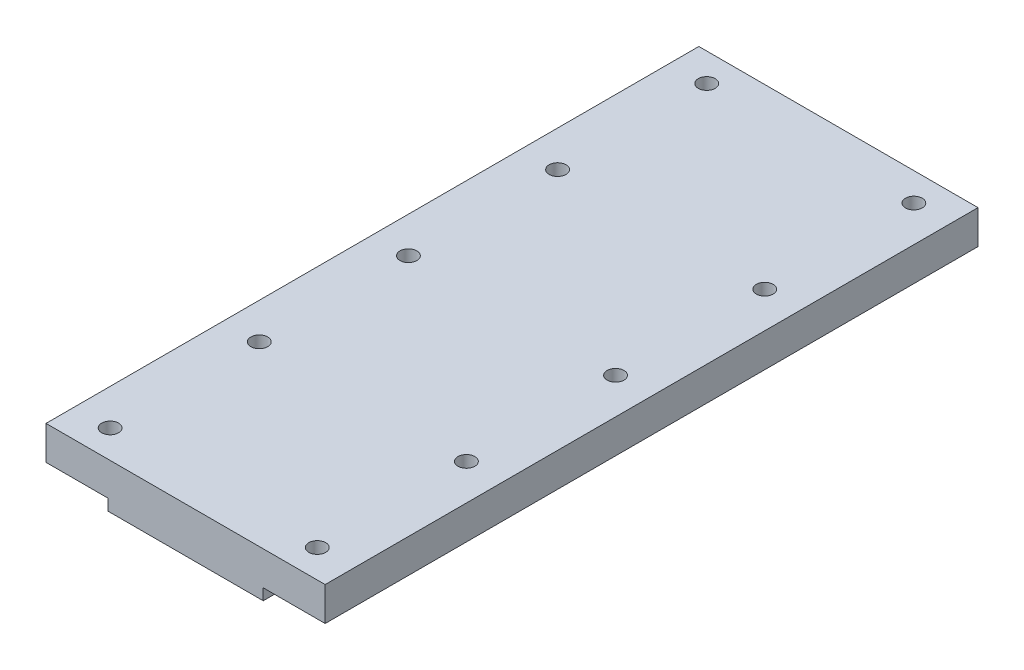
SolidWorks part; units mm, degrees
material "Plain Carbon Steel"
ref_plane "Front Plane" through (0, 0, 0) normal (0, 0, 1) x (1, 0, 0)
ref_plane "Top Plane" through (0, 0, 0) normal (0, 1, 0) x (1, 0, 0)
ref_plane "Right Plane" through (0, 0, 0) normal (1, 0, 0) x (0, 0, -1)
sketch "Plate Profile Sketch" plane through (0, 0, 0) normal (0, 0, 1) x (1, 0, 0)
  line L0 (-124, 0) -> (-69, 0)
  line L1 (-69, 0) -> (-69, -10)
  line L2 (-69, -10) -> (69, -10)
  line L3 (69, -10) -> (69, 0)
  line L4 (69, 0) -> (124, 0)
  line L5 (124, 0) -> (124, 30)
  line L6 (124, 30) -> (-124, 30)
  line L7 (-124, 30) -> (-124, 0)
  line L8 (0, 0) -> (0, 57.2182) construction
  dimension "D1" = 248
  dimension "D2" = 40
  dimension "D3" = 10
  dimension "D4" = 124
  dimension "D5" = 138
extrude "Base Plate" add sketch "Plate Profile Sketch" along normal mid plane 580
sketch "Mounting Holes Sketch" plane through (0, 30, 0) normal (0, 1, 0) x (1, 0, 0)
  line L0 (124, 290) -> (-124, 290) construction
  line L1 (-124, -290) -> (-124, 290) construction
  circle A0 centre (-92, 265) radius 7.5
  circle A1 centre (-92, 132.5) radius 7.5
  circle A2 centre (-92, 0) radius 7.5
  circle A3 centre (-92, -132.5) radius 7.5
  circle A4 centre (-92, -265) radius 7.5
  circle A5 centre (92, 132.5) radius 7.5
  circle A6 centre (92, 0) radius 7.5
  circle A7 centre (92, -132.5) radius 7.5
  circle A8 centre (92, -265) radius 7.5
  circle A9 centre (92, 265) radius 7.5
  dimension "D1" = 15
  dimension "D2" = 25
  dimension "D3" = 92
  dimension "D6" = 216
  dimension "D7" = 157.5
  dimension "D4" = 5
  dimension "D5" = 2
extrude "Mounting Holes 10xØ15" cut sketch "Mounting Holes Sketch" against normal mid plane 580
